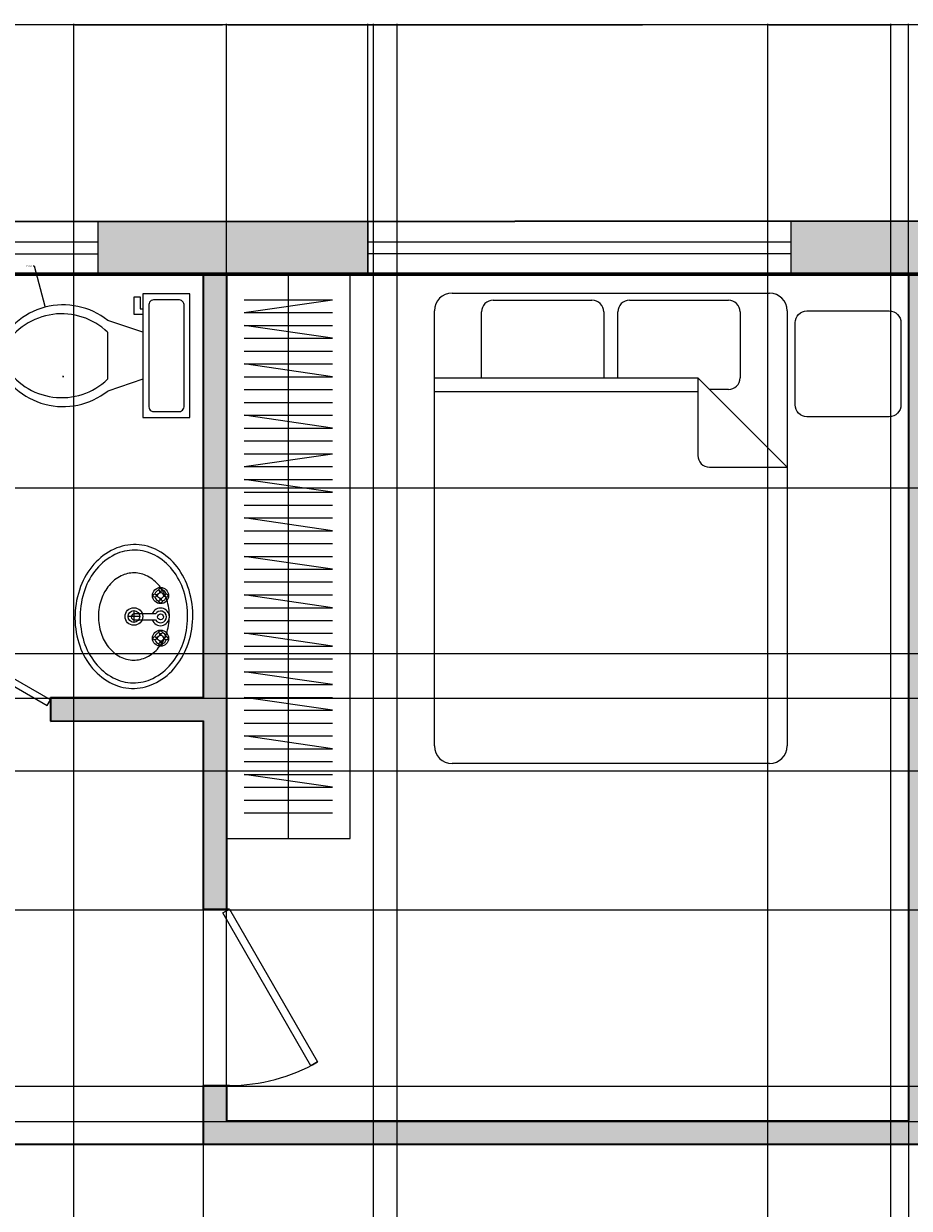
# Model space of a CAD drawing. Units: inches. Extents: x 1531 to 2263, y 2711 to 3216.
# Tile 11 of 12: x 1925 to 2076, y 3015 to 3216. Entities that reach past the tile are written whole.
import ezdxf

# ---------------------------------------------------------------- set-up
doc = ezdxf.new("R2010")
doc.units = ezdxf.units.IN
for name, color, linetype, lineweight in [('A-ANNO-DIMS', 2, 'Continuous', 18), ('A-DOOR', 3, 'Continuous', 25), ('A-FLOR-CASE', 9, 'Continuous', 18), ('A-FLOR-FIXT', 9, 'Continuous', 18), ('A-FURN', 8, 'Continuous', 18), ('A-GLAZ', 4, 'Continuous', 18), ('A-WALL', 7, 'Continuous', 35)]:
    doc.layers.add(name, color=color, linetype=linetype, lineweight=lineweight)
doc.layers.add('A-WALL-PATT', color=18, linetype='Continuous', lineweight=13, true_color=0x000000)
doc.styles.get("Standard").update_dxf_attribs({"font": 'arial.ttf'})
doc.dimstyles.get("Standard").update_dxf_attribs({"dimtxt": 0.18, "dimasz": 0.18, "dimexe": 0.18, "dimexo": 0.0625, "dimgap": 0.09, "dimtad": 0, "dimtih": 1, "dimtoh": 1, "dimdec": 4, "dimzin": 0, "dimdsep": 46, "dimtxsty": 'Standard', "dimcen": 0.09, "dimadec": 0, "dimazin": 0, "dimtfac": 1, "dimtdec": 4, "dimtofl": 0, "dimtmove": 0, "dimatfit": 3, "dimfxl": 1, "dimtolj": 1, "dimtzin": 0, "dimarcsym": 0})

# ---------------------------------------------------------------- blocks, each defined once
blk = doc.blocks.new('*U3')
for p, q in [((0, 0), (0, -6)), ((40, 0), (40, -6))]:
    blk.add_line(p, q)
blk.add_lwpolyline([(0, 0), (34.64, 20), (35.52, 18.48), (0.87, -1.52)], close=True)
blk.add_arc((0, 0), 40, 0, 30)
blk = doc.blocks.new('Toilet - top')
for p, q in [((9.5, -6), (9.5, -2)), ((-8, -8.5), (-8, -8)), ((-7, -8), (-7, -9.5)), ((-4, -8), (-6, -14)), ((4, -8), (6, -14)), ((-10, -8.5), (-8, -8.5)), ((-10, -9.5), (-10, -8.5)), ((-7, -9.5), (-10, -9.5)), ((4, -14), (-4, -14))]:
    blk.add_line(p, q)
blk.add_lwpolyline([(10.5, -8), (10.5, 0), (-10.5, 0), (-10.5, -8)], close=True)
for points in [[(-9.5, -2), (-9.5, -6)], [(8.5, -1), (-8.5, -1)], [(-8.5, -7), (8.5, -7)]]:
    blk.add_lwpolyline(points)
for centre, radius, start, end in [((-8.62, -1.88), 0.884, 81.8699, 188.1301), ((8.62, -1.88), 0.884, 351.8699, 98.1301), ((-8.62, -6.12), 0.884, 171.8699, 278.1301), ((8.62, -6.12), 0.884, 261.8699, 8.1301), ((3.52, -21.58), 12.17, 141.4691, 247.9714), ((4.2, -21.82), 11.33, 136.3677, 238.9468), ((-3.52, -21.58), 12.17, 292.0284, 38.5307), ((-4.2, -21.82), 11.33, 301.053, 43.6321), ((0, -27.88), 4, 245.7318, 294.2682), ((0, -29), 4, 254.8605, 285.1395)]:
    blk.add_arc(centre, radius, start, end)
blk = doc.blocks.new('Sink - Oval top')
for p, q in [((-1, 0), (1, 0)), ((0, 1), (0, -1))]:
    blk.add_line(p, q)
for points in [[(-12.23, 0.39, 0.117634), (-11.46, -3.36, 0.104469), (-8.88, -6.8, 0.090016), (-5.08, -9.07, 0.08192), (-0.32, -10.02, 0.08192), (4.49, -9.38, 0.090016), (8.42, -7.36, 0.104469), (11.22, -4.09, 0.117634), (12.23, -0.39, 0.117634), (11.46, 3.36, 0.104469), (8.88, 6.8, 0.090016), (5.08, 9.07, 0.08192), (0.32, 10.02, 0.08192), (-4.49, 9.38, 0.090016), (-8.42, 7.36, 0.104469), (-11.22, 4.09, 0.117634)], [(-11.29, 0.16, 0.118622), (-10.52, -3.25, 0.104678), (-8.07, -6.36, 0.089562), (-4.54, -8.37, 0.081185), (-0.13, -9.15, 0.081185), (4.3, -8.49, 0.089562), (7.89, -6.58, 0.104678), (10.42, -3.55, 0.118622), (11.29, -0.16, 0.118622), (10.52, 3.25, 0.104678), (8.07, 6.36, 0.089562), (4.54, 8.37, 0.081185), (0.13, 9.15, 0.081185), (-4.3, 8.49, 0.089562), (-7.89, 6.58, 0.104678), (-10.42, 3.55, 0.118622)], [(-7.42, 0.08, 0.118283), (-6.91, -2.17, 0.104607), (-5.29, -4.21, 0.089718), (-2.97, -5.53, 0.081436), (-0.07, -6.04, 0.081436), (2.84, -5.59, 0.089718), (5.2, -4.33, 0.104607), (6.86, -2.32, 0.118283), (7.42, -0.08, 0.118283), (6.91, 2.17, 0.104607), (5.29, 4.21, 0.089718), (2.97, 5.53, 0.081436), (0.07, 6.04, 0.081436), (-2.84, 5.59, 0.089718), (-5.2, 4.33, 0.104607), (-6.86, 2.32, 0.118283)]]:
    blk.add_lwpolyline(points, format="xyb", close=True)
for radius in [1.5, 1]:
    blk.add_circle((0, 0), radius)
blk = doc.blocks.new('Faucet - Bathroom top')
for p, q in [((-4.107, 0.125), (-4.375, 0.125)), ((-3.75, 0.4788), (-3.75, 0.75)), ((-3.5, 0.482), (-3.5, 0.75)), ((-3.1461, 0.125), (-2.875, 0.125)), ((3.143, 0.125), (2.875, 0.125)), ((3.5, 0.4788), (3.5, 0.75)), ((3.75, 0.482), (3.75, 0.75)), ((4.1039, 0.125), (4.375, 0.125)), ((-4.1039, -0.125), (-4.375, -0.125)), ((-3.75, -0.4821), (-3.75, -0.75)), ((-3.5, -0.4789), (-3.5, -0.75)), ((-3.143, -0.125), (-2.875, -0.125)), ((-0.5, -0.8639), (-0.5, -4.5)), ((0.5, -4.5), (0.5, -0.8631)), ((3.1461, -0.125), (2.875, -0.125)), ((3.5, -0.4821), (3.5, -0.75)), ((3.75, -0.4789), (3.75, -0.75)), ((4.107, -0.125), (4.375, -0.125))]:
    blk.add_line(p, q)
for centre, radius in [((-3.625, 0), 1.375), ((-4.625, 0), 0.2795), ((-3.625, 0), 0.5), ((-3.625, 1), 0.2795), ((-2.625, 0), 0.2795), ((0, 0), 0.5), ((3.625, 0), 1.375), ((2.625, 0), 0.2795), ((3.625, 0), 0.5), ((3.625, 1), 0.2795), ((4.625, 0), 0.2795), ((-3.625, -1), 0.2795), ((3.625, -1), 0.2795)]:
    blk.add_circle(centre, radius)
for centre, radius, start, end in [((-3.625, 0), 1, 105.2407, 164.2093), ((-3.625, 0), 1, 16.44125, 74.07887), ((0, 0), 1.5, 289.6514, 250.3603), ((0, 0), 1, 300.3431, 239.7554), ((3.625, 0), 1, 106.12, 164.0884), ((3.625, 0), 1, 16.23422, 73.90469), ((-3.625, 0), 1, 196.2342, 253.9047), ((-3.625, 0), 1, 286.12, 344.0884), ((3.625, 0), 1, 196.4413, 254.0789), ((3.625, 0), 1, 285.2407, 344.2093), ((0, -4.5), 0.5, 180, 0)]:
    blk.add_arc(centre, radius, start, end)
blk = doc.blocks.new('Bed - Queen')
for p, q in [((3, 0), (57, 0)), ((10, -1.2), (26.8, -1.2)), ((33.2, -1.2), (50, -1.2)), ((0, -77), (0, -3)), ((8, -14.4), (8, -3.2)), ((28.8, -3.2), (28.8, -14.4)), ((31.2, -14.4), (31.2, -3.2)), ((52, -3.2), (52, -14.4)), ((60, -3), (60, -77)), ((0, -14.4), (44.8, -14.4)), ((60, -29.6), (44.8, -14.4)), ((44.8, -14.4), (44.8, -27.6)), ((44.8, -16.8), (0, -16.8)), ((50, -16.4), (46.8, -16.4)), ((46.8, -29.6), (60, -29.6)), ((57, -80), (3, -80))]:
    blk.add_line(p, q)
blk.add_lwpolyline([(63.37, -3.02), (77.37, -3.02, -0.414214), (79.37, -5.02), (79.37, -19.02, -0.414214), (77.37, -21.02), (63.37, -21.02, -0.414214), (61.37, -19.02), (61.37, -5.02, -0.414214)], format="xyb", close=True)
for centre, radius, start, end in [((3, -3), 3, 90, 180), ((57, -3), 3, 0, 90), ((10, -3.2), 2, 90, 180), ((26.8, -3.2), 2, 0, 90), ((33.2, -3.2), 2, 90, 180), ((50, -3.2), 2, 0, 90), ((50, -14.4), 2, 270, 0), ((46.8, -27.6), 2, 180, 270), ((3, -77), 3, 180, 270), ((57, -77), 3, 270, 0)]:
    blk.add_arc(centre, radius, start, end)
blk = doc.blocks.new('WIN-72IN')
for p, q in [((0, 5.5), (72, 5.5)), ((0, 3.5), (72, 3.5))]:
    blk.add_line(p, q)
for points in [[(0, 9), (0, 0)], [(72, 0), (72, 9)]]:
    blk.add_lwpolyline(points)
blk = doc.blocks.new('WIN-24IN')
for p, q in [((0, 5.5), (24, 5.5)), ((0, 3.5), (24, 3.5))]:
    blk.add_line(p, q)
for points in [[(0, 9), (0, 0)], [(24, 0), (24, 9)]]:
    blk.add_lwpolyline(points)
blk = doc.blocks.new('WARDROBE-96IN')
for p, q in [((96, 21), (0, 21)), ((0, 21), (0, 0)), ((0, 0), (0, 21)), ((96, 0), (96, 21)), ((4.36, 3), (4.36, 18)), ((6.55, 3), (4.36, 18)), ((6.55, 3), (6.55, 18)), ((8.73, 3), (8.73, 18)), ((10.91, 18), (8.73, 3)), ((10.91, 3), (10.91, 18)), ((13.09, 3), (13.09, 18)), ((15.27, 3), (15.27, 18)), ((17.45, 18), (15.27, 3)), ((17.45, 3), (17.45, 18)), ((19.64, 3), (19.64, 18)), ((21.82, 3), (21.82, 18)), ((24, 3), (24, 18)), ((26.18, 18), (24, 3)), ((26.18, 3), (26.18, 18)), ((28.36, 3), (28.36, 18)), ((30.55, 3), (30.55, 18)), ((32.73, 3), (30.55, 18)), ((32.73, 3), (32.73, 18)), ((34.91, 3), (34.91, 18)), ((37.09, 18), (34.91, 3)), ((37.09, 3), (37.09, 18)), ((39.27, 3), (39.27, 18)), ((41.45, 3), (41.45, 18)), ((43.64, 18), (41.45, 3)), ((43.64, 3), (43.64, 18)), ((45.82, 3), (45.82, 18)), ((48, 3), (48, 18)), ((50.18, 18), (48, 3)), ((50.18, 3), (50.18, 18)), ((52.36, 3), (52.36, 18)), ((54.55, 3), (54.55, 18)), ((56.73, 18), (54.55, 3)), ((56.73, 3), (56.73, 18)), ((58.91, 3), (58.91, 18)), ((61.09, 3), (61.09, 18)), ((63.27, 18), (61.09, 3)), ((63.27, 3), (63.27, 18)), ((65.45, 3), (65.45, 18)), ((67.64, 3), (67.64, 18)), ((69.82, 18), (67.64, 3)), ((69.82, 3), (69.82, 18)), ((72, 3), (72, 18)), ((74.18, 18), (72, 3)), ((74.18, 3), (74.18, 18)), ((76.36, 3), (76.36, 18)), ((78.55, 3), (78.55, 18)), ((80.73, 18), (78.55, 3)), ((80.73, 3), (80.73, 18)), ((82.91, 3), (82.91, 18)), ((85.09, 3), (85.09, 18)), ((87.27, 18), (85.09, 3)), ((87.27, 3), (87.27, 18)), ((89.45, 3), (89.45, 18)), ((91.64, 3), (91.64, 18)), ((96, 10.5), (0, 10.5)), ((0, 0), (96, 0))]:
    blk.add_line(p, q)
blk = doc.blocks.new('*D54')
at = {"layer": 'A-ANNO-DIMS', "color": 0, "lineweight": -2, "transparency": 16777216}
for p, q in [((1568.91, 3182.74), (1568.91, 3216.47)), ((1569.09, 3216.29), (1898.62, 3216.29)), ((2228.73, 3216.29), (1899.2, 3216.29)), ((2228.91, 3183.08), (2228.91, 3216.47))]:
    blk.add_line(p, q, dxfattribs=at)
at = {"layer": 'A-ANNO-DIMS', "color": 0, "transparency": 16777216}
for points in [[(1569.09, 3216.32), (1569.09, 3216.26), (1568.91, 3216.29)], [(2228.73, 3216.32), (2228.73, 3216.26), (2228.91, 3216.29)]]:
    blk.add_solid(points, dxfattribs=at)
at = {"layer": 'Defpoints', "color": 0, "transparency": 16777216}
for p in [(2228.91, 3216.29), (1568.91, 3182.67), (2228.91, 3183.02)]:
    blk.add_point(p, dxfattribs=at)
at = {"layer": 'A-ANNO-DIMS', "color": 0, "transparency": 16777216, "insert": (1898.91, 3216.29), "char_height": 0.18, "attachment_point": 5}
blk.add_mtext('\\A1;660', dxfattribs=at)
blk = doc.blocks.new('*D60')
at = {"layer": 'A-ANNO-DIMS', "color": 0, "lineweight": -2, "transparency": 16777216}
for p, q in [((1899.91, 3097.79), (1899.91, 2711.06)), ((1955.91, 3097.81), (1955.91, 2711.06)), ((1900.09, 2711.24), (1927.69, 2711.24)), ((1955.73, 2711.24), (1928.13, 2711.24))]:
    blk.add_line(p, q, dxfattribs=at)
at = {"layer": 'A-ANNO-DIMS', "color": 0, "transparency": 16777216}
for points in [[(1900.09, 2711.27), (1900.09, 2711.21), (1899.91, 2711.24)], [(1955.73, 2711.27), (1955.73, 2711.21), (1955.91, 2711.24)]]:
    blk.add_solid(points, dxfattribs=at)
at = {"layer": 'Defpoints', "color": 0, "transparency": 16777216}
for p in [(1899.91, 3097.85), (1955.91, 3097.88), (1955.91, 2711.24)]:
    blk.add_point(p, dxfattribs=at)
at = {"layer": 'A-ANNO-DIMS', "color": 0, "transparency": 16777216, "insert": (1927.91, 2711.24), "char_height": 0.18, "attachment_point": 5}
blk.add_mtext('\\A1;56', dxfattribs=at)
blk = doc.blocks.new('*D61')
at = {"layer": 'A-ANNO-DIMS', "color": 0, "lineweight": -2, "transparency": 16777216}
for p, q in [((1959.91, 3029.94), (1959.91, 3216.47)), ((1960.09, 3216.29), (2017.63, 3216.29)), ((2075.73, 3216.29), (2018.19, 3216.29)), ((2075.91, 3030), (2075.91, 3216.47))]:
    blk.add_line(p, q, dxfattribs=at)
at = {"layer": 'A-ANNO-DIMS', "color": 0, "transparency": 16777216}
for points in [[(1960.09, 3216.32), (1960.09, 3216.26), (1959.91, 3216.29)], [(2075.73, 3216.32), (2075.73, 3216.26), (2075.91, 3216.29)]]:
    blk.add_solid(points, dxfattribs=at)
at = {"layer": 'Defpoints', "color": 0, "transparency": 16777216}
for p in [(2075.91, 3216.29), (1959.91, 3029.88), (2075.91, 3029.94)]:
    blk.add_point(p, dxfattribs=at)
at = {"layer": 'A-ANNO-DIMS', "color": 0, "transparency": 16777216, "insert": (2017.91, 3216.29), "char_height": 0.18, "attachment_point": 5}
blk.add_mtext('\\A1;116', dxfattribs=at)
blk = doc.blocks.new('*D71')
at = {"layer": 'A-ANNO-DIMS', "color": 0, "lineweight": -2, "transparency": 16777216}
for p, q in [((1933.91, 2891.93), (1933.91, 3216.47)), ((1934.09, 3216.29), (1959.21, 3216.29)), ((1984.73, 3216.29), (1959.61, 3216.29)), ((1984.91, 2891.95), (1984.91, 3216.47))]:
    blk.add_line(p, q, dxfattribs=at)
at = {"layer": 'A-ANNO-DIMS', "color": 0, "transparency": 16777216}
for points in [[(1934.09, 3216.32), (1934.09, 3216.26), (1933.91, 3216.29)], [(1984.73, 3216.32), (1984.73, 3216.26), (1984.91, 3216.29)]]:
    blk.add_solid(points, dxfattribs=at)
at = {"layer": 'Defpoints', "color": 0, "transparency": 16777216}
for p in [(1984.91, 3216.29), (1933.91, 2891.87), (1984.91, 2891.89)]:
    blk.add_point(p, dxfattribs=at)
at = {"layer": 'A-ANNO-DIMS', "color": 0, "transparency": 16777216, "insert": (1959.41, 3216.29), "char_height": 0.18, "attachment_point": 5}
blk.add_mtext('\\A1;51', dxfattribs=at)
blk = doc.blocks.new('*D79')
at = {"layer": 'A-ANNO-DIMS', "color": 0, "lineweight": -2, "transparency": 16777216}
for p, q in [((1988.91, 2807.93), (1988.91, 3216.47)), ((1989.09, 3216.29), (2030.69, 3216.29)), ((2072.73, 3216.29), (2031.13, 3216.29)), ((2072.91, 2807.93), (2072.91, 3216.47))]:
    blk.add_line(p, q, dxfattribs=at)
at = {"layer": 'A-ANNO-DIMS', "color": 0, "transparency": 16777216}
for points in [[(1989.09, 3216.32), (1989.09, 3216.26), (1988.91, 3216.29)], [(2072.73, 3216.32), (2072.73, 3216.26), (2072.91, 3216.29)]]:
    blk.add_solid(points, dxfattribs=at)
at = {"layer": 'Defpoints', "color": 0, "transparency": 16777216}
for p in [(2072.91, 3216.29), (1988.91, 2807.86), (2072.91, 2807.86)]:
    blk.add_point(p, dxfattribs=at)
at = {"layer": 'A-ANNO-DIMS', "color": 0, "transparency": 16777216, "insert": (2030.91, 3216.29), "char_height": 0.18, "attachment_point": 5}
blk.add_mtext('\\A1;84', dxfattribs=at)
blk = doc.blocks.new('*D80')
at = {"layer": 'A-ANNO-DIMS', "color": 0, "lineweight": -2, "transparency": 16777216}
for p, q in [((1715.97, 3173.75), (2262.37, 3173.75)), ((2262.19, 3173.57), (2262.19, 3137.93)), ((2262.19, 3101.93), (2262.19, 3137.57)), ((1715.97, 3101.75), (2262.37, 3101.75))]:
    blk.add_line(p, q, dxfattribs=at)
at = {"layer": 'A-ANNO-DIMS', "color": 0, "transparency": 16777216}
for points in [[(2262.16, 3173.57), (2262.22, 3173.57), (2262.19, 3173.75)], [(2262.16, 3101.93), (2262.22, 3101.93), (2262.19, 3101.75)]]:
    blk.add_solid(points, dxfattribs=at)
at = {"layer": 'Defpoints', "color": 0, "transparency": 16777216}
for p in [(1715.91, 3173.75), (1715.91, 3101.75), (2262.19, 3101.75)]:
    blk.add_point(p, dxfattribs=at)
at = {"layer": 'A-ANNO-DIMS', "color": 0, "transparency": 16777216, "insert": (2262.19, 3137.75), "char_height": 0.18, "attachment_point": 5}
blk.add_mtext('\\A1;72', dxfattribs=at)
blk = doc.blocks.new('*D85')
at = {"layer": 'A-ANNO-DIMS', "color": 0, "lineweight": -2, "transparency": 16777216}
for p, q in [((2079.85, 3173.94), (1531.04, 3173.94)), ((1531.22, 3173.76), (1531.22, 3131.82)), ((1531.22, 3089.52), (1531.22, 3131.46)), ((2079.85, 3089.34), (1531.04, 3089.34))]:
    blk.add_line(p, q, dxfattribs=at)
at = {"layer": 'A-ANNO-DIMS', "color": 0, "transparency": 16777216}
for points in [[(1531.19, 3173.76), (1531.25, 3173.76), (1531.22, 3173.94)], [(1531.19, 3089.52), (1531.25, 3089.52), (1531.22, 3089.34)]]:
    blk.add_solid(points, dxfattribs=at)
at = {"layer": 'Defpoints', "color": 0, "transparency": 16777216}
for p in [(1531.22, 3173.94), (2079.91, 3173.94), (2079.91, 3089.34)]:
    blk.add_point(p, dxfattribs=at)
at = {"layer": 'A-ANNO-DIMS', "color": 0, "transparency": 16777216, "insert": (1531.22, 3131.64), "char_height": 0.18, "attachment_point": 5}
blk.add_mtext('\\A1;84.6', dxfattribs=at)
blk = doc.blocks.new('*D86')
at = {"layer": 'A-ANNO-DIMS', "color": 0, "lineweight": -2, "transparency": 16777216}
for p, q in [((1715.97, 3065.75), (2262.37, 3065.75)), ((2262.19, 3065.57), (2262.19, 3050.93)), ((2262.19, 3035.93), (2262.19, 3050.57)), ((1715.97, 3035.75), (2262.37, 3035.75))]:
    blk.add_line(p, q, dxfattribs=at)
at = {"layer": 'A-ANNO-DIMS', "color": 0, "transparency": 16777216}
for points in [[(2262.16, 3065.57), (2262.22, 3065.57), (2262.19, 3065.75)], [(2262.16, 3035.93), (2262.22, 3035.93), (2262.19, 3035.75)]]:
    blk.add_solid(points, dxfattribs=at)
at = {"layer": 'Defpoints', "color": 0, "transparency": 16777216}
for p in [(1715.91, 3065.75), (2262.19, 3065.75), (1715.91, 3035.75)]:
    blk.add_point(p, dxfattribs=at)
at = {"layer": 'A-ANNO-DIMS', "color": 0, "transparency": 16777216, "insert": (2262.19, 3050.75), "char_height": 0.18, "attachment_point": 5}
blk.add_mtext('\\A1;30', dxfattribs=at)
blk = doc.blocks.new('*D92')
at = {"layer": 'A-ANNO-DIMS', "color": 0, "lineweight": -2, "transparency": 16777216}
for p, q in [((1959.91, 3173.94), (1959.91, 3216.47)), ((1960.09, 3216.29), (1971.54, 3216.29)), ((1983.78, 3216.29), (1972.33, 3216.29)), ((1983.96, 3173.95), (1983.96, 3216.47))]:
    blk.add_line(p, q, dxfattribs=at)
at = {"layer": 'A-ANNO-DIMS', "color": 0, "transparency": 16777216}
for points in [[(1960.09, 3216.32), (1960.09, 3216.26), (1959.91, 3216.29)], [(1983.78, 3216.32), (1983.78, 3216.26), (1983.96, 3216.29)]]:
    blk.add_solid(points, dxfattribs=at)
at = {"layer": 'Defpoints', "color": 0, "transparency": 16777216}
for p in [(1983.96, 3216.29), (1959.91, 3173.88), (1983.96, 3173.89)]:
    blk.add_point(p, dxfattribs=at)
at = {"layer": 'A-ANNO-DIMS', "color": 0, "transparency": 16777216, "insert": (1971.93, 3216.29), "char_height": 0.18, "attachment_point": 5}
blk.add_mtext('\\A1;24.05', dxfattribs=at)
blk = doc.blocks.new('*D100')
at = {"layer": 'A-ANNO-DIMS', "color": 0, "lineweight": -2, "transparency": 16777216}
for p, q in [((2219.85, 3174.02), (1531.04, 3174.02)), ((1531.22, 3173.84), (1531.22, 3155.93)), ((1531.22, 3137.67), (1531.22, 3155.57)), ((2219.85, 3137.49), (1531.04, 3137.49))]:
    blk.add_line(p, q, dxfattribs=at)
at = {"layer": 'A-ANNO-DIMS', "color": 0, "transparency": 16777216}
for points in [[(1531.19, 3173.84), (1531.25, 3173.84), (1531.22, 3174.02)], [(1531.19, 3137.67), (1531.25, 3137.67), (1531.22, 3137.49)]]:
    blk.add_solid(points, dxfattribs=at)
at = {"layer": 'Defpoints', "color": 0, "transparency": 16777216}
for p in [(2219.91, 3174.02), (1531.22, 3137.49), (2219.91, 3137.49)]:
    blk.add_point(p, dxfattribs=at)
at = {"layer": 'A-ANNO-DIMS', "color": 0, "transparency": 16777216, "insert": (1531.22, 3155.75), "char_height": 0.18, "attachment_point": 5}
blk.add_mtext('\\A1;36.526', dxfattribs=at)
blk = doc.blocks.new('*D103')
at = {"layer": 'A-ANNO-DIMS', "color": 0, "lineweight": -2, "transparency": 16777216}
for p, q in [((1577.97, 3173.68), (2262.37, 3173.68)), ((2262.19, 3173.5), (2262.19, 3141.71)), ((2262.19, 3109.55), (2262.19, 3141.34)), ((1577.97, 3109.37), (2262.37, 3109.37))]:
    blk.add_line(p, q, dxfattribs=at)
at = {"layer": 'A-ANNO-DIMS', "color": 0, "transparency": 16777216}
for points in [[(2262.16, 3173.5), (2262.22, 3173.5), (2262.19, 3173.68)], [(2262.16, 3109.55), (2262.22, 3109.55), (2262.19, 3109.37)]]:
    blk.add_solid(points, dxfattribs=at)
at = {"layer": 'Defpoints', "color": 0, "transparency": 16777216}
for p in [(1577.91, 3173.68), (1577.91, 3109.37), (2262.19, 3109.37)]:
    blk.add_point(p, dxfattribs=at)
at = {"layer": 'A-ANNO-DIMS', "color": 0, "transparency": 16777216, "insert": (2262.19, 3141.52), "char_height": 0.18, "attachment_point": 5}
blk.add_mtext('\\A1;64.31', dxfattribs=at)
blk = doc.blocks.new('*D110')
at = {"layer": 'A-ANNO-DIMS', "color": 0, "lineweight": -2, "transparency": 16777216}
for p, q in [((1711.97, 3035.75), (2262.37, 3035.75)), ((2262.19, 3035.57), (2262.19, 3032.93)), ((2262.19, 3029.93), (2262.19, 3032.57)), ((1711.97, 3029.75), (2262.37, 3029.75))]:
    blk.add_line(p, q, dxfattribs=at)
at = {"layer": 'A-ANNO-DIMS', "color": 0, "transparency": 16777216}
for points in [[(2262.16, 3035.57), (2262.22, 3035.57), (2262.19, 3035.75)], [(2262.16, 3029.93), (2262.22, 3029.93), (2262.19, 3029.75)]]:
    blk.add_solid(points, dxfattribs=at)
at = {"layer": 'Defpoints', "color": 0, "transparency": 16777216}
for p in [(1711.91, 3035.75), (2262.19, 3035.75), (1711.91, 3029.75)]:
    blk.add_point(p, dxfattribs=at)
at = {"layer": 'A-ANNO-DIMS', "color": 0, "transparency": 16777216, "insert": (2262.19, 3032.75), "char_height": 0.18, "attachment_point": 5}
blk.add_mtext('\\A1;6', dxfattribs=at)
blk = doc.blocks.new('*D116')
at = {"layer": 'A-ANNO-DIMS', "color": 0, "lineweight": -2, "transparency": 16777216}
for p, q in [((1899.97, 3025.85), (2262.37, 3025.85)), ((2262.19, 3025.67), (2262.19, 3014.79)), ((2262.19, 3003.56), (2262.19, 3014.43)), ((1894.62, 3003.38), (2262.37, 3003.38))]:
    blk.add_line(p, q, dxfattribs=at)
at = {"layer": 'A-ANNO-DIMS', "color": 0, "transparency": 16777216}
for points in [[(2262.16, 3025.67), (2262.22, 3025.67), (2262.19, 3025.85)], [(2262.16, 3003.56), (2262.22, 3003.56), (2262.19, 3003.38)]]:
    blk.add_solid(points, dxfattribs=at)
at = {"layer": 'Defpoints', "color": 0, "transparency": 16777216}
for p in [(1899.91, 3025.85), (1894.55, 3003.38), (2262.19, 3003.38)]:
    blk.add_point(p, dxfattribs=at)
at = {"layer": 'A-ANNO-DIMS', "color": 0, "transparency": 16777216, "insert": (2262.19, 3014.61), "char_height": 0.18, "attachment_point": 5}
blk.add_mtext('\\A1;22.47', dxfattribs=at)
blk = doc.blocks.new('*D121')
at = {"layer": 'A-ANNO-DIMS', "color": 0, "lineweight": -2, "transparency": 16777216}
for p, q in [((2052, 2979.08), (2052, 3216.47)), ((2052.18, 3216.29), (2073.04, 3216.29)), ((2094.69, 3216.29), (2073.83, 3216.29)), ((2094.87, 2979.39), (2094.87, 3216.47))]:
    blk.add_line(p, q, dxfattribs=at)
at = {"layer": 'A-ANNO-DIMS', "color": 0, "transparency": 16777216}
for points in [[(2052.18, 3216.32), (2052.18, 3216.26), (2052, 3216.29)], [(2094.69, 3216.32), (2094.69, 3216.26), (2094.87, 3216.29)]]:
    blk.add_solid(points, dxfattribs=at)
at = {"layer": 'Defpoints', "color": 0, "transparency": 16777216}
for p in [(2094.87, 3216.29), (2052, 2979.01), (2094.87, 2979.33)]:
    blk.add_point(p, dxfattribs=at)
at = {"layer": 'A-ANNO-DIMS', "color": 0, "transparency": 16777216, "insert": (2073.43, 3216.29), "char_height": 0.18, "attachment_point": 5}
blk.add_mtext('\\A1;42.87', dxfattribs=at)
blk = doc.blocks.new('*D122')
at = {"layer": 'A-ANNO-DIMS', "color": 0, "lineweight": -2, "transparency": 16777216}
for p, q in [((1955.85, 3025.88), (1531.04, 3025.88)), ((1531.22, 3025.7), (1531.22, 3009.49)), ((1531.22, 2992.91), (1531.22, 3009.12)), ((1968.31, 2992.73), (1531.04, 2992.73))]:
    blk.add_line(p, q, dxfattribs=at)
at = {"layer": 'A-ANNO-DIMS', "color": 0, "transparency": 16777216}
for points in [[(1531.19, 3025.7), (1531.25, 3025.7), (1531.22, 3025.88)], [(1531.19, 2992.91), (1531.25, 2992.91), (1531.22, 2992.73)]]:
    blk.add_solid(points, dxfattribs=at)
at = {"layer": 'Defpoints', "color": 0, "transparency": 16777216}
for p in [(1531.22, 3025.88), (1955.91, 3025.88), (1968.37, 2992.73)]:
    blk.add_point(p, dxfattribs=at)
at = {"layer": 'A-ANNO-DIMS', "color": 0, "transparency": 16777216, "insert": (1531.22, 3009.3), "char_height": 0.18, "attachment_point": 5}
blk.add_mtext('\\A1;33.146', dxfattribs=at)
blk = doc.blocks.new('*D130')
at = {"layer": 'A-ANNO-DIMS', "color": 0, "lineweight": -2, "transparency": 16777216}
for p, q in [((2075.91, 3029.88), (2075.91, 2711.06)), ((2079.91, 3025.88), (2079.91, 2711.06)), ((2076.09, 2711.24), (2077.76, 2711.24)), ((2079.73, 2711.24), (2078.06, 2711.24))]:
    blk.add_line(p, q, dxfattribs=at)
at = {"layer": 'A-ANNO-DIMS', "color": 0, "transparency": 16777216}
for points in [[(2076.09, 2711.27), (2076.09, 2711.21), (2075.91, 2711.24)], [(2079.73, 2711.27), (2079.73, 2711.21), (2079.91, 2711.24)]]:
    blk.add_solid(points, dxfattribs=at)
at = {"layer": 'Defpoints', "color": 0, "transparency": 16777216}
for p in [(2075.91, 3029.94), (2079.91, 3025.94), (2075.91, 2711.24)]:
    blk.add_point(p, dxfattribs=at)
at = {"layer": 'A-ANNO-DIMS', "color": 0, "transparency": 16777216, "insert": (2077.91, 2711.24), "char_height": 0.18, "attachment_point": 5}
blk.add_mtext('\\A1;4', dxfattribs=at)
blk = doc.blocks.new('*D132')
at = {"layer": 'A-ANNO-DIMS', "color": 0, "lineweight": -2, "transparency": 16777216}
for p, q in [((1926.96, 3175.31), (1927.14, 3175.31)), ((1927.14, 3175.31), (1928.95, 3168.43)), ((1932, 3156.48), (1932.18, 3156.48)), ((1932.09, 3156.39), (1932.09, 3156.57))]:
    blk.add_line(p, q, dxfattribs=at)
at = {"layer": 'A-ANNO-DIMS', "color": 0, "transparency": 16777216}
blk.add_solid([(1928.98, 3168.43), (1928.92, 3168.42), (1928.99, 3168.25)], dxfattribs=at)
at = {"layer": 'Defpoints', "color": 0, "transparency": 16777216}
for p in [(1928.99, 3168.25), (1932.09, 3156.48)]:
    blk.add_point(p, dxfattribs=at)
at = {"layer": 'A-ANNO-DIMS', "color": 0, "transparency": 16777216, "insert": (1926.29, 3175.31), "char_height": 0.18, "attachment_point": 5}
blk.add_mtext('\\A1;8X R12.17', dxfattribs=at)

msp = doc.modelspace()

# ---------------------------------------------------------------- hatches: boundary and pattern name
at = {"layer": 'A-WALL-PATT'}
h = msp.add_hatch(color=256, dxfattribs=at)
h.dxf.hatch_style = 1
h.paths.add_polyline_path([(1983.9596, 3182.8919), (1938.0228, 3182.8679), (1938.0228, 3173.8679), (1955.9101, 3173.8772), (1955.9101, 3101.8772), (1929.9101, 3101.8636), (1929.9101, 3097.8636), (1955.9101, 3097.8772), (1955.9101, 3065.8772), (1959.9101, 3065.8793), (1959.9101, 3173.8793), (1983.9596, 3173.8919)])
h = msp.add_hatch(color=256, dxfattribs=at)
h.dxf.hatch_style = 1
h.paths.add_polyline_path([(2228.9101, 3183.02), (2055.9596, 3182.9296), (2055.9596, 3173.9296), (2075.9101, 3173.94), (2075.9101, 3029.94), (1959.9101, 3029.8793), (1959.9101, 3035.8772), (1955.9101, 3035.8772), (1955.9101, 3025.8772), (2079.9101, 3025.9421), (2079.9101, 3173.9421), (2219.9101, 3174.0153), (2219.9101, 3137.4897), (2228.9101, 3137.4897)])

# ---------------------------------------------------------------- linework, layer by layer
at = {"layer": 'A-WALL'}
for p, q in [((1899.9101, 3173.8479), (1955.9101, 3173.8772)), ((1955.9101, 3173.8772), (1955.9101, 3101.8772)), ((1959.9101, 3173.8793), (2075.9101, 3173.94)), ((1959.9101, 3173.8793), (1959.9101, 3065.8793)), ((2075.9101, 3173.94), (2075.9101, 3029.94)), ((1929.9101, 3101.8636), (1955.9101, 3101.8772)), ((1929.9101, 3101.8636), (1929.9101, 3097.8479)), ((1929.9101, 3097.8636), (1955.9101, 3097.8772)), ((1955.9101, 3097.8772), (1955.9101, 3065.8772)), ((1955.8913, 3065.8772), (1959.9101, 3065.8793)), ((1955.907, 3035.8772), (1959.9101, 3035.8793)), ((1955.9101, 3035.8772), (1955.9101, 3025.8772)), ((1959.9101, 3035.8793), (1959.9101, 3029.8793)), ((1959.9101, 3029.8793), (2075.9101, 3029.94)), ((1955.9101, 3025.8772), (2079.9101, 3025.9421))]:
    msp.add_line(p, q, dxfattribs=at)
msp.add_lwpolyline([(1933.9101, 2762.8657), (1568.9111, 2762.6748), (1568.9111, 3182.6749), (2228.9101, 3183.02), (2228.9101, 2798.8631)], dxfattribs=at)

# ---------------------------------------------------------------- block references
at = {"layer": 'A-DOOR', "xscale": -0.6, "yscale": 0.6, "zscale": 0.6}
msp.add_blockref('*U3', (1929.9101, 3101.4479), dxfattribs=at)
at = {"layer": 'A-DOOR', "xscale": 0.75, "yscale": 0.75, "zscale": 0.75, "rotation": 270}
msp.add_blockref('*U3', (1960.3913, 3065.8772), dxfattribs=at)
at = {"layer": 'A-FLOR-CASE', "rotation": 269.9999999999949}
msp.add_blockref('WARDROBE-96IN', (1959.9106, 3173.8794), dxfattribs=at)
at = {"layer": 'A-FLOR-FIXT', "rotation": 270}
for name, p in [('Toilet - top', (1953.6666, 3160.0021)), ('Sink - Oval top', (1944.1271, 3115.6498)), ('Faucet - Bathroom top', (1948.6639, 3115.5821))]:
    msp.add_blockref(name, p, dxfattribs=at)
at = {"layer": 'A-FURN'}
msp.add_blockref('Bed - Queen', (1995.2774, 3170.6455), dxfattribs=at)
at = {"layer": 'A-GLAZ'}
for name, p in [('WIN-24IN', (1914.023, 3173.855)), ('WIN-72IN', (1983.9597, 3173.8918))]:
    msp.add_blockref(name, p, dxfattribs=at)

# ---------------------------------------------------------------- dimensions: what is measured, and where the dimension line sits
at = {"layer": 'A-ANNO-DIMS'}
for base, p1, p2, override, picture, middle in [((2228.9101, 3216.295), (1568.9111, 3182.6749), (2228.9101, 3183.02), {"dimdec": 0, "dimlfac": 1, "dimrnd": 0, "dimzin": 0, "dimdsep": 46, "dimlunit": 2}, '*D54', (1898.9106, 3216.295)), ((1984.9101, 3216.295), (1933.9101, 2891.8657), (1984.9101, 2891.8924), {"dimdec": 0, "dimlfac": 1, "dimrnd": 0, "dimzin": 0, "dimdsep": 46, "dimlunit": 2}, '*D71', (1959.4101, 3216.295)), ((2075.9101, 3216.295), (1959.9101, 3029.8793), (2075.9101, 3029.94), {"dimdec": 0, "dimlfac": 1, "dimrnd": 0, "dimzin": 0, "dimdsep": 46, "dimlunit": 2}, '*D61', (2017.9101, 3216.295)), ((1983.9596, 3216.295), (1959.9101, 3173.8793), (1983.9596, 3173.8919), {"dimdec": 2, "dimlfac": 1, "dimrnd": 0, "dimzin": 0, "dimdsep": 46, "dimlunit": 2}, '*D92', (1971.9349, 3216.295)), ((2072.9101, 3216.295), (1988.9101, 2807.8631), (2072.9101, 2807.8631), {"dimdec": 0, "dimlfac": 1, "dimrnd": 0, "dimzin": 0, "dimdsep": 46, "dimlunit": 2}, '*D79', (2030.9101, 3216.295)), ((2094.8704, 3216.295), (2051.9983, 2979.0128), (2094.8704, 2979.3315), {"dimdec": 2, "dimlfac": 1, "dimrnd": 0, "dimzin": 0, "dimdsep": 46, "dimlunit": 2}, '*D121', (2073.4343, 3216.295)), ((1955.9101, 2711.2407), (1899.9101, 3097.8479), (1955.9101, 3097.8772), {"dimdec": 0, "dimlfac": 1, "dimrnd": 0, "dimzin": 0, "dimdsep": 46, "dimlunit": 2}, '*D60', (1927.9101, 2711.2407)), ((2075.9101, 2711.2407), (2079.9101, 3025.9421), (2075.9101, 3029.94), {"dimdec": 0, "dimlfac": 1, "dimrnd": 0, "dimzin": 0, "dimdsep": 46, "dimlunit": 2}, '*D130', (2077.9101, 2711.2407))]:
    dim = msp.add_linear_dim(base=base, p1=p1, p2=p2, dimstyle='Standard', override=override, dxfattribs=at)
    dim.commit()
    dim.dimension.update_dxf_attribs({"geometry": picture, "text_midpoint": middle})
dim = msp.add_radius_dim(center=(1932.0861, 3156.4825), mpoint=(1928.994, 3168.2521), text='8X <>', dimstyle='Standard', override={"dimdec": 2, "dimlfac": 1, "dimrnd": 0, "dimzin": 0, "dimdsep": 46, "dimlunit": 2}, dxfattribs=at)
dim.commit()
dim.dimension.update_dxf_attribs({"geometry": '*D132', "text_midpoint": (1926.2853, 3175.3139), "dimtype": 164})
for base, p1, p2, override, picture, middle in [((1531.2212, 3137.4897), (2219.9101, 3174.0153), (2219.9101, 3137.4897), {"dimdec": 3, "dimlfac": 1, "dimrnd": 0, "dimzin": 0, "dimdsep": 46, "dimlunit": 2}, '*D100', (1531.2212, 3155.7525)), ((1531.2212, 3173.9421), (2079.9101, 3089.343), (2079.9101, 3173.9421), {"dimdec": 1, "dimlfac": 1, "dimrnd": 0, "dimzin": 0, "dimdsep": 46, "dimlunit": 2}, '*D85', (1531.2212, 3131.6425)), ((2262.1851, 3109.3695), (1577.9111, 3173.6796), (1577.9111, 3109.3695), {"dimdec": 2, "dimlfac": 1, "dimrnd": 0, "dimzin": 0, "dimdsep": 46, "dimlunit": 2}, '*D103', (2262.1851, 3141.5245)), ((2262.1851, 3101.7517), (1715.9101, 3173.7517), (1715.9101, 3101.7517), {"dimdec": 0, "dimlfac": 1, "dimrnd": 0, "dimzin": 0, "dimdsep": 46, "dimlunit": 2}, '*D80', (2262.1851, 3137.7517)), ((2262.1851, 3065.7517), (1715.9101, 3035.7517), (1715.9101, 3065.7517), {"dimdec": 0, "dimlfac": 1, "dimrnd": 0, "dimzin": 0, "dimdsep": 46, "dimlunit": 2}, '*D86', (2262.1851, 3050.7517)), ((2262.1851, 3035.7496), (1711.9101, 3029.7496), (1711.9101, 3035.7496), {"dimdec": 0, "dimlfac": 1, "dimrnd": 0, "dimzin": 0, "dimdsep": 46, "dimlunit": 2}, '*D110', (2262.1851, 3032.7496)), ((1531.2212, 3025.8772), (1968.3722, 2992.7314), (1955.9101, 3025.8772), {"dimdec": 3, "dimlfac": 1, "dimrnd": 0, "dimzin": 0, "dimdsep": 46, "dimlunit": 2}, '*D122', (1531.2212, 3009.3043)), ((2262.1851, 3003.376), (1899.9101, 3025.8479), (1894.5532, 3003.376), {"dimdec": 2, "dimlfac": 1, "dimrnd": 0, "dimzin": 0, "dimdsep": 46, "dimlunit": 2}, '*D116', (2262.1851, 3014.6119))]:
    dim = msp.add_linear_dim(base=base, p1=p1, p2=p2, angle=90, dimstyle='Standard', override=override, dxfattribs=at)
    dim.commit()
    dim.dimension.update_dxf_attribs({"geometry": picture, "text_midpoint": middle})

doc.saveas('drawing.dxf')
